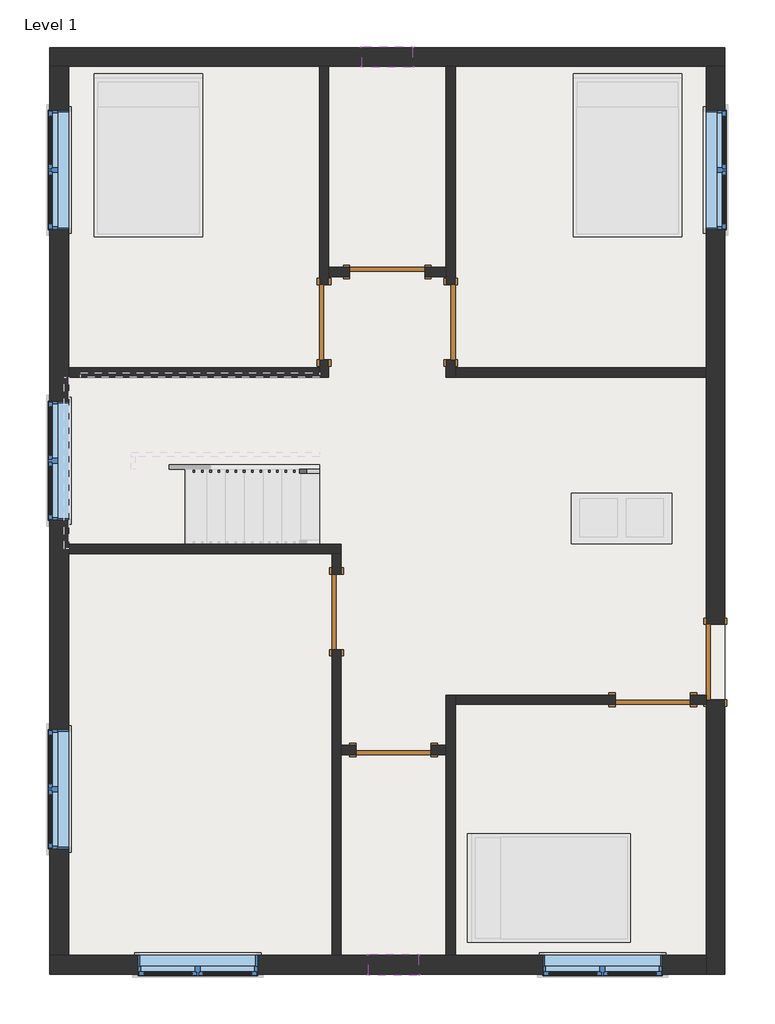
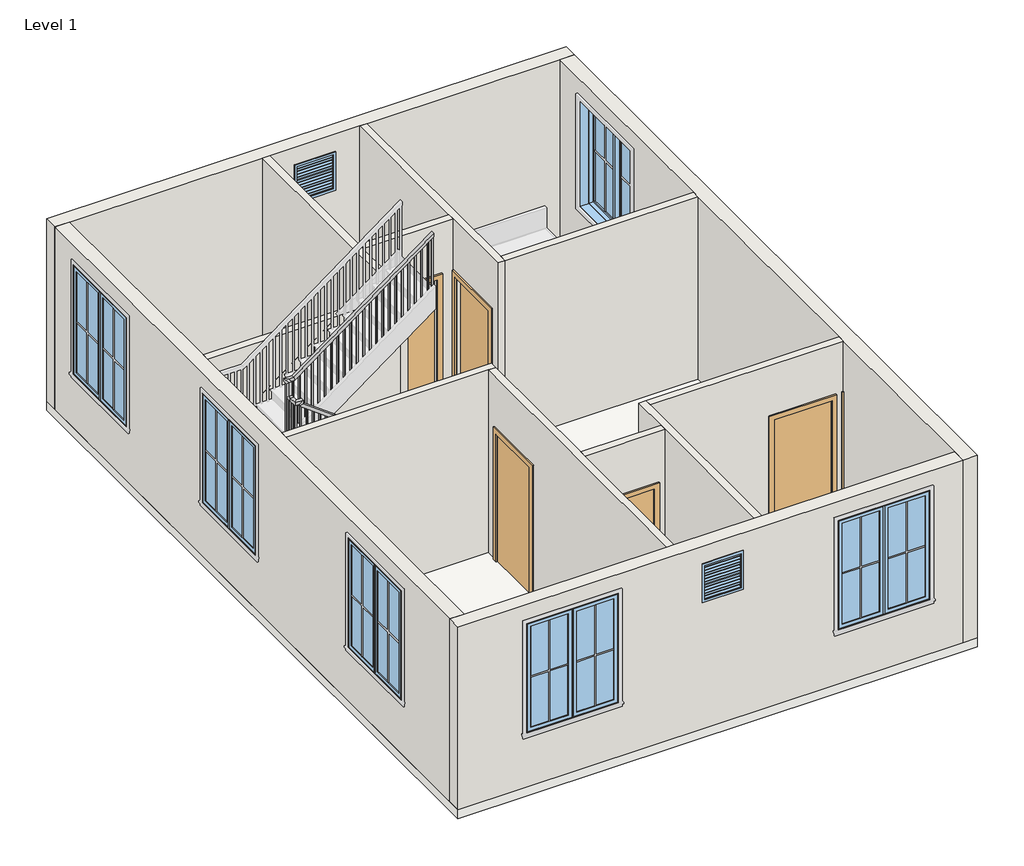
# One storey, part 1 of 2: 14 walls, 8 windows, 7 doors, 1 railing, 1 slab.
"""IFC4 building model written with IfcOpenShell, lengths in millimetres."""

from ifc_helpers import new_model, si_unit, frame, origin, origin_with_axes, place, context, project, spatial, polyline, outline, extrude, faceted_brep, transform, mapped, element, save
from components import door_305aa2a5, door_e5f9f3c4, door_0ca8825f, window_9ac97e1a, window_f2d8fef0

model = new_model("IFC4")

# Units and contexts
model_context = context("Model", 3, world=origin())
ifc_project = project(units=[si_unit("LENGTHUNIT", "METRE", prefix="MILLI")], contexts=[model_context])

# Site, building, storey
site = spatial("IfcSite", under=ifc_project)
building = spatial("IfcBuilding", under=site)
storey = spatial("IfcBuildingStorey", under=building, Name="Level 1", Elevation=0.0)

# Doors
placement = place(None, origin())
door_shape = door_305aa2a5(model_context)
element("IfcDoor", 1, ObjectType="Single-Flush : 36\" x 84\"", at=placement, inside=storey, context=model_context, shape_type="MappedRepresentation", body=[
    mapped(door_shape, transform((-2023.6910855, 2116.5303617, 0.0), x_axis=(0.0, -1.0, 0.0), y_axis=(1.0, 0.0, 0.0), z_axis=(0.0, 0.0, 1.0))),
])
element("IfcDoor", 2, ObjectType="Single-Flush : 36\" x 84\"", at=placement, inside=storey, context=model_context, shape_type="MappedRepresentation", body=[
    mapped(door_shape, transform((-1179.1410855, -3078.1725945, 0.0), x_axis=(1.0, 0.0, 0.0), y_axis=(0.0, 1.0, 0.0), z_axis=(0.0, 0.0, 1.0))),
])
element("IfcDoor", 3, ObjectType="Single-Flush : 36\" x 84\"", at=placement, inside=storey, context=model_context, shape_type="MappedRepresentation", body=[
    mapped(door_shape, transform((1970.4589145, -2468.1696383, 0.0), x_axis=(1.0, 0.0, 0.0), y_axis=(0.0, 1.0, 0.0), z_axis=(0.0, 0.0, 1.0))),
])
door_2_shape = door_e5f9f3c4(model_context)
element("IfcDoor", 4, ObjectType="Single-Flush : 36\" x 84\"", at=placement, inside=storey, context=model_context, shape_type="MappedRepresentation", body=[
    mapped(door_2_shape, transform((-486.9910855, 2116.5303617, 0.0), x_axis=(0.0, -1.0, 0.0), y_axis=(1.0, 0.0, 0.0), z_axis=(0.0, 0.0, 1.0))),
])
element("IfcDoor", 5, ObjectType="Single-Flush : 36\" x 84\"", at=placement, inside=storey, context=model_context, shape_type="MappedRepresentation", body=[
    mapped(door_2_shape, transform((-1871.2910855, -1401.3696383, 0.0), x_axis=(0.0, 1.0, 0.0), y_axis=(-1.0, 0.0, 0.0), z_axis=(0.0, 0.0, 1.0))),
])
element("IfcDoor", 6, ObjectType="Single-Flush : 36\" x 84\"", at=placement, inside=storey, context=model_context, shape_type="MappedRepresentation", body=[
    mapped(door_2_shape, transform((-1255.3410855, 2726.1303617, 0.0), x_axis=(1.0, 0.0, 0.0), y_axis=(0.0, 1.0, 0.0), z_axis=(0.0, 0.0, 1.0))),
])
door_3_shape = door_0ca8825f(model_context)
element("IfcDoor", 7, ObjectType="Single-Flush : 36\" x 84\"", at=placement, inside=storey, context=model_context, shape_type="MappedRepresentation", body=[
    mapped(door_3_shape, transform((2732.4589145, -2010.9696383, 0.0), x_axis=(0.0, 1.0, 0.0), y_axis=(-1.0, 0.0, 0.0), z_axis=(0.0, 0.0, 1.0))),
])

# Railing
element("IfcRailing", 8, ObjectType="Handrail - Rectangular", at=placement, inside=storey, context=model_context, shape_type="SolidModel", body=[
    faceted_brep([(-2080.8410855, 281.3803617, 1083.7333333), (-2080.8410855, 281.3803617, 1020.5144356), (-2080.8410855, 332.1803617, 1020.5144356), (-2080.8410855, 332.1803617, 1083.7333333), (-4290.6410855, 281.3803617, 2720.6222222), (-4341.4410855, 281.3803617, 2695.0329542), (-4341.4410855, 332.1803617, 2695.0329542), (-4290.6410855, 332.1803617, 2720.6222222), (-4290.6410855, 281.3803617, 2777.0666667), (-4341.4410855, 281.3803617, 2726.2666667), (-4341.4410855, 332.1803617, 2726.2666667), (-4290.6410855, 332.1803617, 2777.0666667), (-4417.6410855, 281.3803617, 2777.0666667), (-4417.6410855, 281.3803617, 2726.2666667), (-4366.8410855, 332.1803617, 2726.2666667), (-4366.8410855, 332.1803617, 2777.0666667), (-4417.6410855, 408.3803617, 2777.0666667), (-4417.6410855, 408.3803617, 2726.2666667), (-4366.8410855, 408.3803617, 2726.2666667), (-4366.8410855, 408.3803617, 2777.0666667), (-4417.6410855, 459.1803617, 2777.0666667), (-4417.6410855, 509.9803617, 2726.2666667), (-4366.8410855, 509.9803617, 2726.2666667), (-4366.8410855, 459.1803617, 2777.0666667), (-4417.6410855, 459.1803617, 3002.8444444), (-4417.6410855, 509.9803617, 2952.0444444), (-4366.8410855, 509.9803617, 2952.0444444), (-4366.8410855, 459.1803617, 3002.8444444), (-4417.6410855, 586.1803617, 3002.8444444), (-4417.6410855, 586.1803617, 2952.0444444), (-4366.8410855, 535.3803617, 2952.0444444), (-4366.8410855, 535.3803617, 3002.8444444), (-4290.6410855, 586.1803617, 3002.8444444), (-4273.8755736, 586.1803617, 2952.0444444), (-4273.8755736, 535.3803617, 2952.0444444), (-4290.6410855, 535.3803617, 3002.8444444), (-2080.8410855, 586.1803617, 4639.7333333), (-2080.8410855, 535.3803617, 4639.7333333), (-2080.8410855, 535.3803617, 4576.5144356), (-2080.8410855, 586.1803617, 4576.5144356)], [[[0, 1, 2, 3]], [[1, 0, 4, 5]], [[2, 1, 5, 6]], [[3, 2, 6, 7]], [[0, 3, 7, 4]], [[5, 4, 8, 9]], [[6, 5, 9, 10]], [[7, 6, 10, 11]], [[4, 7, 11, 8]], [[9, 8, 12, 13]], [[10, 9, 13, 14]], [[11, 10, 14, 15]], [[8, 11, 15, 12]], [[13, 12, 16, 17]], [[14, 13, 17, 18]], [[15, 14, 18, 19]], [[12, 15, 19, 16]], [[17, 16, 20, 21]], [[18, 17, 21, 22]], [[19, 18, 22, 23]], [[16, 19, 23, 20]], [[21, 20, 24, 25]], [[22, 21, 25, 26]], [[23, 22, 26, 27]], [[20, 23, 27, 24]], [[25, 24, 28, 29]], [[26, 25, 29, 30]], [[27, 26, 30, 31]], [[24, 27, 31, 28]], [[29, 28, 32, 33]], [[30, 29, 33, 34]], [[31, 30, 34, 35]], [[28, 31, 35, 32]], [[36, 37, 38, 39]], [[33, 32, 36, 39]], [[34, 33, 39, 38]], [[35, 34, 38, 37]], [[32, 35, 37, 36]]]),
    extrude(outline(polyline([(4527.1255467, -2147.5160855), (4513.0144356, -2166.5660855), (3556.0, -2166.5660855), (3556.0, -2147.5160855), (4527.1255467, -2147.5160855)])), frame((0.0, 551.2553617, 0.0), z_axis=(0.0, 1.0, 0.0), x_axis=(0.0, 0.0, 1.0)), (0.0, 0.0, 1.0), 19.05),
    extrude(outline(polyline([(4451.8662875, -2249.1160855), (4437.7551764, -2268.1660855), (3556.0, -2268.1660855), (3556.0, -2249.1160855), (4451.8662875, -2249.1160855)])), frame((0.0, 551.2553617, 0.0), z_axis=(0.0, 1.0, 0.0), x_axis=(0.0, 0.0, 1.0)), (0.0, 0.0, 1.0), 19.05),
    extrude(outline(polyline([(4376.6070282, -2350.7160855), (4362.4959171, -2369.7660855), (3386.6666667, -2369.7660855), (3386.6666667, -2350.7160855), (4376.6070282, -2350.7160855)])), frame((0.0, 551.2553617, 0.0), z_axis=(0.0, 1.0, 0.0), x_axis=(0.0, 0.0, 1.0)), (0.0, 0.0, 1.0), 19.05),
    extrude(outline(polyline([(4301.347769, -2452.3160855), (4287.2366579, -2471.3660855), (3386.6666667, -2471.3660855), (3386.6666667, -2452.3160855), (4301.347769, -2452.3160855)])), frame((0.0, 551.2553617, 0.0), z_axis=(0.0, 1.0, 0.0), x_axis=(0.0, 0.0, 1.0)), (0.0, 0.0, 1.0), 19.05),
    extrude(outline(polyline([(4226.0885097, -2553.9160855), (4211.9773986, -2572.9660855), (3217.3333333, -2572.9660855), (3217.3333333, -2553.9160855), (4226.0885097, -2553.9160855)])), frame((0.0, 551.2553617, 0.0), z_axis=(0.0, 1.0, 0.0), x_axis=(0.0, 0.0, 1.0)), (0.0, 0.0, 1.0), 19.05),
    extrude(outline(polyline([(4150.8292505, -2655.5160855), (4136.7181393, -2674.5660855), (3217.3333333, -2674.5660855), (3217.3333333, -2655.5160855), (4150.8292505, -2655.5160855)])), frame((0.0, 551.2553617, 0.0), z_axis=(0.0, 1.0, 0.0), x_axis=(0.0, 0.0, 1.0)), (0.0, 0.0, 1.0), 19.05),
    extrude(outline(polyline([(4075.5699912, -2757.1160855), (4061.4588801, -2776.1660855), (3217.3333333, -2776.1660855), (3217.3333333, -2757.1160855), (4075.5699912, -2757.1160855)])), frame((0.0, 551.2553617, 0.0), z_axis=(0.0, 1.0, 0.0), x_axis=(0.0, 0.0, 1.0)), (0.0, 0.0, 1.0), 19.05),
    extrude(outline(polyline([(4000.3107319, -2858.7160855), (3986.1996208, -2877.7660855), (3048.0, -2877.7660855), (3048.0, -2858.7160855), (4000.3107319, -2858.7160855)])), frame((0.0, 551.2553617, 0.0), z_axis=(0.0, 1.0, 0.0), x_axis=(0.0, 0.0, 1.0)), (0.0, 0.0, 1.0), 19.05),
    extrude(outline(polyline([(3925.0514727, -2960.3160855), (3910.9403616, -2979.3660855), (3048.0, -2979.3660855), (3048.0, -2960.3160855), (3925.0514727, -2960.3160855)])), frame((0.0, 551.2553617, 0.0), z_axis=(0.0, 1.0, 0.0), x_axis=(0.0, 0.0, 1.0)), (0.0, 0.0, 1.0), 19.05),
    extrude(outline(polyline([(3849.7922134, -3061.9160855), (3835.6811023, -3080.9660855), (2878.6666667, -3080.9660855), (2878.6666667, -3061.9160855), (3849.7922134, -3061.9160855)])), frame((0.0, 551.2553617, 0.0), z_axis=(0.0, 1.0, 0.0), x_axis=(0.0, 0.0, 1.0)), (0.0, 0.0, 1.0), 19.05),
    extrude(outline(polyline([(3774.5329542, -3163.5160855), (3760.421843, -3182.5660855), (2878.6666667, -3182.5660855), (2878.6666667, -3163.5160855), (3774.5329542, -3163.5160855)])), frame((0.0, 551.2553617, 0.0), z_axis=(0.0, 1.0, 0.0), x_axis=(0.0, 0.0, 1.0)), (0.0, 0.0, 1.0), 19.05),
    extrude(outline(polyline([(3699.2736949, -3265.1160855), (3685.1625838, -3284.1660855), (2709.3333333, -3284.1660855), (2709.3333333, -3265.1160855), (3699.2736949, -3265.1160855)])), frame((0.0, 551.2553617, 0.0), z_axis=(0.0, 1.0, 0.0), x_axis=(0.0, 0.0, 1.0)), (0.0, 0.0, 1.0), 19.05),
    extrude(outline(polyline([(3624.0144356, -3366.7160855), (3609.9033245, -3385.7660855), (2709.3333333, -3385.7660855), (2709.3333333, -3366.7160855), (3624.0144356, -3366.7160855)])), frame((0.0, 551.2553617, 0.0), z_axis=(0.0, 1.0, 0.0), x_axis=(0.0, 0.0, 1.0)), (0.0, 0.0, 1.0), 19.05),
    extrude(outline(polyline([(3548.7551764, -3468.3160855), (3534.6440653, -3487.3660855), (2540.0, -3487.3660855), (2540.0, -3468.3160855), (3548.7551764, -3468.3160855)])), frame((0.0, 551.2553617, 0.0), z_axis=(0.0, 1.0, 0.0), x_axis=(0.0, 0.0, 1.0)), (0.0, 0.0, 1.0), 19.05),
    extrude(outline(polyline([(3473.4959171, -3569.9160855), (3459.384806, -3588.9660855), (2540.0, -3588.9660855), (2540.0, -3569.9160855), (3473.4959171, -3569.9160855)])), frame((0.0, 551.2553617, 0.0), z_axis=(0.0, 1.0, 0.0), x_axis=(0.0, 0.0, 1.0)), (0.0, 0.0, 1.0), 19.05),
    extrude(outline(polyline([(3398.2366579, -3671.5160855), (3384.1255467, -3690.5660855), (2540.0, -3690.5660855), (2540.0, -3671.5160855), (3398.2366579, -3671.5160855)])), frame((0.0, 551.2553617, 0.0), z_axis=(0.0, 1.0, 0.0), x_axis=(0.0, 0.0, 1.0)), (0.0, 0.0, 1.0), 19.05),
    extrude(outline(polyline([(3322.9773986, -3773.1160855), (3308.8662875, -3792.1660855), (2370.6666667, -3792.1660855), (2370.6666667, -3773.1160855), (3322.9773986, -3773.1160855)])), frame((0.0, 551.2553617, 0.0), z_axis=(0.0, 1.0, 0.0), x_axis=(0.0, 0.0, 1.0)), (0.0, 0.0, 1.0), 19.05),
    extrude(outline(polyline([(3247.7181393, -3874.7160855), (3233.6070282, -3893.7660855), (2370.6666667, -3893.7660855), (2370.6666667, -3874.7160855), (3247.7181393, -3874.7160855)])), frame((0.0, 551.2553617, 0.0), z_axis=(0.0, 1.0, 0.0), x_axis=(0.0, 0.0, 1.0)), (0.0, 0.0, 1.0), 19.05),
    extrude(outline(polyline([(3172.4588801, -3976.3160855), (3158.347769, -3995.3660855), (2201.3333333, -3995.3660855), (2201.3333333, -3976.3160855), (3172.4588801, -3976.3160855)])), frame((0.0, 551.2553617, 0.0), z_axis=(0.0, 1.0, 0.0), x_axis=(0.0, 0.0, 1.0)), (0.0, 0.0, 1.0), 19.05),
    extrude(outline(polyline([(3097.1996208, -4077.9160855), (3083.0885097, -4096.9660855), (2201.3333333, -4096.9660855), (2201.3333333, -4077.9160855), (3097.1996208, -4077.9160855)])), frame((0.0, 551.2553617, 0.0), z_axis=(0.0, 1.0, 0.0), x_axis=(0.0, 0.0, 1.0)), (0.0, 0.0, 1.0), 19.05),
    extrude(outline(polyline([(3021.9403616, -4179.5160855), (3007.8292505, -4198.5660855), (2032.0, -4198.5660855), (2032.0, -4179.5160855), (3021.9403616, -4179.5160855)])), frame((0.0, 551.2553617, 0.0), z_axis=(0.0, 1.0, 0.0), x_axis=(0.0, 0.0, 1.0)), (0.0, 0.0, 1.0), 19.05),
    extrude(outline(polyline([(2946.6811023, -4281.1160855), (2932.5699912, -4300.1660855), (2032.0, -4300.1660855), (2032.0, -4281.1160855), (2946.6811023, -4281.1160855)])), frame((0.0, 551.2553617, 0.0), z_axis=(0.0, 1.0, 0.0), x_axis=(0.0, 0.0, 1.0)), (0.0, 0.0, 1.0), 19.05),
    extrude(outline(polyline([(-4382.7160855, 500.4553617), (-4401.7660855, 500.4553617), (-4401.7660855, 519.5053617), (-4382.7160855, 519.5053617), (-4382.7160855, 500.4553617)])), frame((0.0, 0.0, 1862.6666667), z_axis=(0.0, 0.0, 1.0), x_axis=(1.0, 0.0, 0.0)), (0.0, 0.0, 1.0), 1089.3777778),
    extrude(outline(polyline([(-4382.7160855, 398.8553617), (-4401.7660855, 398.8553617), (-4401.7660855, 417.9053617), (-4382.7160855, 417.9053617), (-4382.7160855, 398.8553617)])), frame((0.0, 0.0, 1862.6666667), z_axis=(0.0, 0.0, 1.0), x_axis=(1.0, 0.0, 0.0)), (0.0, 0.0, 1.0), 863.6),
    extrude(outline(polyline([(-4306.5160855, 316.3053617), (-4306.5160855, 297.2553617), (-4325.5660855, 297.2553617), (-4325.5660855, 316.3053617), (-4306.5160855, 316.3053617)])), frame((0.0, 0.0, 1693.3333333), z_axis=(0.0, 0.0, 1.0), x_axis=(1.0, 0.0, 0.0)), (0.0, 0.0, 1.0), 1032.9333333),
    extrude(outline(polyline([(2593.9033245, -4204.9160855), (2608.0144356, -4223.9660855), (1693.3333333, -4223.9660855), (1693.3333333, -4204.9160855), (2593.9033245, -4204.9160855)])), frame((0.0, 297.2553617, 0.0), z_axis=(0.0, 1.0, 0.0), x_axis=(0.0, 0.0, 1.0)), (0.0, 0.0, 1.0), 19.05),
    extrude(outline(polyline([(2518.6440653, -4103.3160855), (2532.7551764, -4122.3660855), (1524.0, -4122.3660855), (1524.0, -4103.3160855), (2518.6440653, -4103.3160855)])), frame((0.0, 297.2553617, 0.0), z_axis=(0.0, 1.0, 0.0), x_axis=(0.0, 0.0, 1.0)), (0.0, 0.0, 1.0), 19.05),
    extrude(outline(polyline([(2443.384806, -4001.7160855), (2457.4959171, -4020.7660855), (1524.0, -4020.7660855), (1524.0, -4001.7160855), (2443.384806, -4001.7160855)])), frame((0.0, 297.2553617, 0.0), z_axis=(0.0, 1.0, 0.0), x_axis=(0.0, 0.0, 1.0)), (0.0, 0.0, 1.0), 19.05),
    extrude(outline(polyline([(2368.1255467, -3900.1160855), (2382.2366579, -3919.1660855), (1524.0, -3919.1660855), (1524.0, -3900.1160855), (2368.1255467, -3900.1160855)])), frame((0.0, 297.2553617, 0.0), z_axis=(0.0, 1.0, 0.0), x_axis=(0.0, 0.0, 1.0)), (0.0, 0.0, 1.0), 19.05),
    extrude(outline(polyline([(2292.8662875, -3798.5160855), (2306.9773986, -3817.5660855), (1354.6666667, -3817.5660855), (1354.6666667, -3798.5160855), (2292.8662875, -3798.5160855)])), frame((0.0, 297.2553617, 0.0), z_axis=(0.0, 1.0, 0.0), x_axis=(0.0, 0.0, 1.0)), (0.0, 0.0, 1.0), 19.05),
    extrude(outline(polyline([(2217.6070282, -3696.9160855), (2231.7181393, -3715.9660855), (1354.6666667, -3715.9660855), (1354.6666667, -3696.9160855), (2217.6070282, -3696.9160855)])), frame((0.0, 297.2553617, 0.0), z_axis=(0.0, 1.0, 0.0), x_axis=(0.0, 0.0, 1.0)), (0.0, 0.0, 1.0), 19.05),
    extrude(outline(polyline([(2142.347769, -3595.3160855), (2156.4588801, -3614.3660855), (1185.3333333, -3614.3660855), (1185.3333333, -3595.3160855), (2142.347769, -3595.3160855)])), frame((0.0, 297.2553617, 0.0), z_axis=(0.0, 1.0, 0.0), x_axis=(0.0, 0.0, 1.0)), (0.0, 0.0, 1.0), 19.05),
    extrude(outline(polyline([(2067.0885097, -3493.7160855), (2081.1996208, -3512.7660855), (1185.3333333, -3512.7660855), (1185.3333333, -3493.7160855), (2067.0885097, -3493.7160855)])), frame((0.0, 297.2553617, 0.0), z_axis=(0.0, 1.0, 0.0), x_axis=(0.0, 0.0, 1.0)), (0.0, 0.0, 1.0), 19.05),
    extrude(outline(polyline([(1991.8292505, -3392.1160855), (2005.9403616, -3411.1660855), (1016.0, -3411.1660855), (1016.0, -3392.1160855), (1991.8292505, -3392.1160855)])), frame((0.0, 297.2553617, 0.0), z_axis=(0.0, 1.0, 0.0), x_axis=(0.0, 0.0, 1.0)), (0.0, 0.0, 1.0), 19.05),
    extrude(outline(polyline([(1916.5699912, -3290.5160855), (1930.6811023, -3309.5660855), (1016.0, -3309.5660855), (1016.0, -3290.5160855), (1916.5699912, -3290.5160855)])), frame((0.0, 297.2553617, 0.0), z_axis=(0.0, 1.0, 0.0), x_axis=(0.0, 0.0, 1.0)), (0.0, 0.0, 1.0), 19.05),
    extrude(outline(polyline([(1841.3107319, -3188.9160855), (1855.421843, -3207.9660855), (846.6666667, -3207.9660855), (846.6666667, -3188.9160855), (1841.3107319, -3188.9160855)])), frame((0.0, 297.2553617, 0.0), z_axis=(0.0, 1.0, 0.0), x_axis=(0.0, 0.0, 1.0)), (0.0, 0.0, 1.0), 19.05),
    extrude(outline(polyline([(1766.0514727, -3087.3160855), (1780.1625838, -3106.3660855), (846.6666667, -3106.3660855), (846.6666667, -3087.3160855), (1766.0514727, -3087.3160855)])), frame((0.0, 297.2553617, 0.0), z_axis=(0.0, 1.0, 0.0), x_axis=(0.0, 0.0, 1.0)), (0.0, 0.0, 1.0), 19.05),
    extrude(outline(polyline([(1690.7922134, -2985.7160855), (1704.9033245, -3004.7660855), (846.6666667, -3004.7660855), (846.6666667, -2985.7160855), (1690.7922134, -2985.7160855)])), frame((0.0, 297.2553617, 0.0), z_axis=(0.0, 1.0, 0.0), x_axis=(0.0, 0.0, 1.0)), (0.0, 0.0, 1.0), 19.05),
    extrude(outline(polyline([(1615.5329542, -2884.1160855), (1629.6440653, -2903.1660855), (677.3333333, -2903.1660855), (677.3333333, -2884.1160855), (1615.5329542, -2884.1160855)])), frame((0.0, 297.2553617, 0.0), z_axis=(0.0, 1.0, 0.0), x_axis=(0.0, 0.0, 1.0)), (0.0, 0.0, 1.0), 19.05),
    extrude(outline(polyline([(1540.2736949, -2782.5160855), (1554.384806, -2801.5660855), (677.3333333, -2801.5660855), (677.3333333, -2782.5160855), (1540.2736949, -2782.5160855)])), frame((0.0, 297.2553617, 0.0), z_axis=(0.0, 1.0, 0.0), x_axis=(0.0, 0.0, 1.0)), (0.0, 0.0, 1.0), 19.05),
    extrude(outline(polyline([(1465.0144356, -2680.9160855), (1479.1255467, -2699.9660855), (508.0, -2699.9660855), (508.0, -2680.9160855), (1465.0144356, -2680.9160855)])), frame((0.0, 297.2553617, 0.0), z_axis=(0.0, 1.0, 0.0), x_axis=(0.0, 0.0, 1.0)), (0.0, 0.0, 1.0), 19.05),
    extrude(outline(polyline([(1389.7551764, -2579.3160855), (1403.8662875, -2598.3660855), (508.0, -2598.3660855), (508.0, -2579.3160855), (1389.7551764, -2579.3160855)])), frame((0.0, 297.2553617, 0.0), z_axis=(0.0, 1.0, 0.0), x_axis=(0.0, 0.0, 1.0)), (0.0, 0.0, 1.0), 19.05),
    extrude(outline(polyline([(1314.4959171, -2477.7160855), (1328.6070282, -2496.7660855), (338.6666667, -2496.7660855), (338.6666667, -2477.7160855), (1314.4959171, -2477.7160855)])), frame((0.0, 297.2553617, 0.0), z_axis=(0.0, 1.0, 0.0), x_axis=(0.0, 0.0, 1.0)), (0.0, 0.0, 1.0), 19.05),
    extrude(outline(polyline([(1239.2366579, -2376.1160855), (1253.347769, -2395.1660855), (338.6666667, -2395.1660855), (338.6666667, -2376.1160855), (1239.2366579, -2376.1160855)])), frame((0.0, 297.2553617, 0.0), z_axis=(0.0, 1.0, 0.0), x_axis=(0.0, 0.0, 1.0)), (0.0, 0.0, 1.0), 19.05),
    extrude(outline(polyline([(1163.9773986, -2274.5160855), (1178.0885097, -2293.5660855), (169.3333333, -2293.5660855), (169.3333333, -2274.5160855), (1163.9773986, -2274.5160855)])), frame((0.0, 297.2553617, 0.0), z_axis=(0.0, 1.0, 0.0), x_axis=(0.0, 0.0, 1.0)), (0.0, 0.0, 1.0), 19.05),
    extrude(outline(polyline([(1088.7181393, -2172.9160855), (1102.8292505, -2191.9660855), (169.3333333, -2191.9660855), (169.3333333, -2172.9160855), (1088.7181393, -2172.9160855)])), frame((0.0, 297.2553617, 0.0), z_axis=(0.0, 1.0, 0.0), x_axis=(0.0, 0.0, 1.0)), (0.0, 0.0, 1.0), 19.05),
    extrude(outline(polyline([(-4382.7160855, 551.2553617), (-4401.7660855, 551.2553617), (-4401.7660855, 570.3053617), (-4382.7160855, 570.3053617), (-4382.7160855, 551.2553617)])), frame((0.0, 0.0, 1862.6666667), z_axis=(0.0, 0.0, 1.0), x_axis=(1.0, 0.0, 0.0)), (0.0, 0.0, 1.0), 1089.3777778),
    extrude(outline(polyline([(-4382.7160855, 316.3053617), (-4382.7160855, 297.2553617), (-4401.7660855, 297.2553617), (-4401.7660855, 316.3053617), (-4382.7160855, 316.3053617)])), frame((0.0, 0.0, 1862.6666667), z_axis=(0.0, 0.0, 1.0), x_axis=(1.0, 0.0, 0.0)), (0.0, 0.0, 1.0), 863.6),
    extrude(outline(polyline([(4576.5144356, -2080.8410855), (4562.4033245, -2099.8910855), (3556.0, -2099.8910855), (3556.0, -2080.8410855), (4576.5144356, -2080.8410855)])), frame((0.0, 551.2553617, 0.0), z_axis=(0.0, 1.0, 0.0), x_axis=(0.0, 0.0, 1.0)), (0.0, 0.0, 1.0), 19.05),
    extrude(outline(polyline([(1020.5144356, -2080.8410855), (1034.6255467, -2099.8910855), (169.3333333, -2099.8910855), (169.3333333, -2080.8410855), (1020.5144356, -2080.8410855)])), frame((0.0, 297.2553617, 0.0), z_axis=(0.0, 1.0, 0.0), x_axis=(0.0, 0.0, 1.0)), (0.0, 0.0, 1.0), 19.05),
])

# Slab
element("IfcSlab", 9, ObjectType="FLOOR 6\"", at=placement, inside=storey, context=model_context, shape_type="SweptSolid", body=[
    extrude(outline(polyline([(2846.7589145, 5450.2803617), (2846.7589145, -5801.9196383), (-5357.4410855, -5801.9196383), (-5357.4410855, 5450.2803617), (2846.7589145, 5450.2803617)])), frame((0.0, 0.0, -152.4), z_axis=(0.0, 0.0, 1.0), x_axis=(1.0, 0.0, 0.0)), (0.0, 0.0, 1.0), 152.4),
])

# Walls
element("IfcWall", 10, ObjectType="WALL 4.5\"", at=placement, inside=storey, context=model_context, shape_type="Brep", body=[
    faceted_brep([(-2080.8410855, 1659.3303617, 2133.6), (-2080.8410855, 1659.3303617, 0.0), (-2080.8410855, 1564.0803617, 0.0), (-2080.8410855, 1449.7803617, 0.0), (-2080.8410855, 1449.7803617, 3048.0), (-2080.8410855, 1564.0803617, 3048.0), (-2080.8410855, 5221.6803617, 3048.0), (-2080.8410855, 5221.6803617, 0.0), (-2080.8410855, 2573.7303617, 0.0), (-2080.8410855, 2573.7303617, 2133.6), (-1966.5410855, 1449.7803617, 0.0), (-1966.5410855, 1659.3303617, 0.0), (-1966.5410855, 1659.3303617, 2133.6), (-1966.5410855, 2573.7303617, 2133.6), (-1966.5410855, 2573.7303617, 0.0), (-1966.5410855, 2668.9803617, 0.0), (-1966.5410855, 2783.2803617, 0.0), (-1966.5410855, 5221.6803617, 0.0), (-1966.5410855, 5221.6803617, 3048.0), (-1966.5410855, 2783.2803617, 3048.0), (-1966.5410855, 2668.9803617, 3048.0), (-1966.5410855, 1449.7803617, 3048.0)], [[[0, 1, 2, 3, 4, 5, 6, 7, 8, 9]], [[10, 11, 12, 13, 14, 15, 16, 17, 18, 19, 20, 21]], [[8, 7, 17, 16, 15, 14]], [[3, 2, 1, 11, 10]], [[7, 6, 18, 17]], [[4, 3, 10, 21]], [[12, 11, 1, 0]], [[13, 12, 0, 9]], [[14, 13, 9, 8]], [[6, 5, 4, 21, 20, 19, 18]]]),
])
element("IfcWall", 11, ObjectType="WALL 4.5\"", at=placement, inside=storey, context=model_context, shape_type="SweptSolid", body=[
    extrude(outline(polyline([(-5128.8410855, 1564.0803617), (-2080.8410855, 1564.0803617), (-2080.8410855, 1449.7803617), (-5128.8410855, 1449.7803617), (-5128.8410855, 1564.0803617)])), origin_with_axes(), (0.0, 0.0, 1.0), 3048.0),
])
element("IfcWall", 12, ObjectType="WALL 4.5\"", at=placement, inside=storey, context=model_context, shape_type="Brep", body=[
    faceted_brep([(-544.1410855, 1659.3303617, 2133.6), (-544.1410855, 1659.3303617, 0.0), (-544.1410855, 1449.7803617, 0.0), (-544.1410855, 1449.7803617, 3048.0), (-544.1410855, 2668.9803617, 3048.0), (-544.1410855, 2783.2803617, 3048.0), (-544.1410855, 5221.6803617, 3048.0), (-544.1410855, 5221.6803617, 0.0), (-544.1410855, 2783.2803617, 0.0), (-544.1410855, 2668.9803617, 0.0), (-544.1410855, 2573.7303617, 0.0), (-544.1410855, 2573.7303617, 2133.6), (-429.8410855, 1449.7803617, 0.0), (-429.8410855, 1564.0803617, 0.0), (-429.8410855, 1659.3303617, 0.0), (-429.8410855, 1659.3303617, 2133.6), (-429.8410855, 2573.7303617, 2133.6), (-429.8410855, 2573.7303617, 0.0), (-429.8410855, 5221.6803617, 0.0), (-429.8410855, 5221.6803617, 3048.0), (-429.8410855, 1564.0803617, 3048.0), (-429.8410855, 1449.7803617, 3048.0)], [[[0, 1, 2, 3, 4, 5, 6, 7, 8, 9, 10, 11]], [[12, 13, 14, 15, 16, 17, 18, 19, 20, 21]], [[2, 1, 14, 13, 12]], [[10, 9, 8, 7, 18, 17]], [[7, 6, 19, 18]], [[3, 2, 12, 21]], [[15, 14, 1, 0]], [[16, 15, 0, 11]], [[17, 16, 11, 10]], [[6, 5, 4, 3, 21, 20, 19]]]),
])
element("IfcWall", 13, ObjectType="WALL 4.5\"", at=placement, inside=storey, context=model_context, shape_type="SweptSolid", body=[
    extrude(outline(polyline([(2618.1589145, 1449.7803617), (-429.8410855, 1449.7803617), (-429.8410855, 1564.0803617), (2618.1589145, 1564.0803617), (2618.1589145, 1449.7803617)])), origin_with_axes(), (0.0, 0.0, 1.0), 3048.0),
])
element("IfcWall", 14, ObjectType="WALL 4.5\"", at=placement, inside=storey, context=model_context, shape_type="Brep", body=[
    faceted_brep([(-5128.8410855, -696.5196383, 0.0), (-1928.4410855, -696.5196383, 0.0), (-1814.1410855, -696.5196383, 0.0), (-1814.1410855, -696.5196383, 3048.0), (-1928.4410855, -696.5196383, 3048.0), (-5128.8410855, -696.5196383, 3048.0), (-5128.8410855, -582.2196383, 0.0), (-5128.8410855, -582.2196383, 3048.0), (-1814.1410855, -582.2196383, 3048.0), (-1814.1410855, -582.2196383, 0.0)], [[[0, 1, 2, 3, 4, 5]], [[6, 7, 8, 9]], [[2, 1, 0, 6, 9]], [[0, 5, 7, 6]], [[3, 2, 9, 8]], [[5, 4, 3, 8, 7]]]),
])
element("IfcWall", 15, ObjectType="WALL 4.5\"", at=placement, inside=storey, context=model_context, shape_type="Brep", body=[
    faceted_brep([(-1814.1410855, -944.1696383, 2133.6), (-1814.1410855, -944.1696383, 0.0), (-1814.1410855, -696.5196383, 0.0), (-1814.1410855, -696.5196383, 3048.0), (-1814.1410855, -3021.0225945, 3048.0), (-1814.1410855, -3135.3225945, 3048.0), (-1814.1410855, -5573.3196383, 3048.0), (-1814.1410855, -5573.3196383, 0.0), (-1814.1410855, -3135.3225945, 0.0), (-1814.1410855, -3021.0225945, 0.0), (-1814.1410855, -1858.5696383, 0.0), (-1814.1410855, -1858.5696383, 2133.6), (-1928.4410855, -696.5196383, 0.0), (-1928.4410855, -944.1696383, 0.0), (-1928.4410855, -944.1696383, 2133.6), (-1928.4410855, -1858.5696383, 2133.6), (-1928.4410855, -1858.5696383, 0.0), (-1928.4410855, -5573.3196383, 0.0), (-1928.4410855, -5573.3196383, 3048.0), (-1928.4410855, -696.5196383, 3048.0)], [[[0, 1, 2, 3, 4, 5, 6, 7, 8, 9, 10, 11]], [[12, 13, 14, 15, 16, 17, 18, 19]], [[2, 1, 13, 12]], [[10, 9, 8, 7, 17, 16]], [[3, 2, 12, 19]], [[7, 6, 18, 17]], [[14, 13, 1, 0]], [[15, 14, 0, 11]], [[16, 15, 11, 10]], [[6, 5, 4, 3, 19, 18]]]),
])
element("IfcWall", 16, ObjectType="WALL 4.5\"", at=placement, inside=storey, context=model_context, shape_type="SweptSolid", body=[
    extrude(outline(polyline([(2133.6, -721.9410855), (0.0, -721.9410855), (0.0, -544.1410855), (3048.0, -544.1410855), (3048.0, -1814.1410855), (0.0, -1814.1410855), (0.0, -1636.3410855), (2133.6, -1636.3410855), (2133.6, -721.9410855)])), frame((0.0, -3135.3225945, 0.0), z_axis=(0.0, 1.0, 0.0), x_axis=(0.0, 0.0, 1.0)), (0.0, 0.0, 1.0), 114.3),
])
element("IfcWall", 17, ObjectType="WALL 4.5\"", at=placement, inside=storey, context=model_context, shape_type="Brep", body=[
    faceted_brep([(-544.1410855, -2411.0196383, 0.0), (-544.1410855, -3021.0225945, 0.0), (-544.1410855, -3135.3225945, 0.0), (-544.1410855, -5573.3196383, 0.0), (-544.1410855, -5573.3196383, 3048.0), (-544.1410855, -3135.3225945, 3048.0), (-544.1410855, -3021.0225945, 3048.0), (-544.1410855, -2411.0196383, 3048.0), (-429.8410855, -2411.0196383, 0.0), (-429.8410855, -2411.0196383, 3048.0), (-429.8410855, -2525.3196383, 3048.0), (-429.8410855, -5573.3196383, 3048.0), (-429.8410855, -5573.3196383, 0.0), (-429.8410855, -2525.3196383, 0.0)], [[[0, 1, 2, 3, 4, 5, 6, 7]], [[8, 9, 10, 11, 12, 13]], [[3, 2, 1, 0, 8, 13, 12]], [[4, 3, 12, 11]], [[0, 7, 9, 8]], [[7, 6, 5, 4, 11, 10, 9]]]),
])
element("IfcWall", 18, ObjectType="WALL 4.5\"", at=placement, inside=storey, context=model_context, shape_type="Brep", body=[
    faceted_brep([(2427.6589145, -2525.3196383, 2133.6), (2427.6589145, -2525.3196383, 0.0), (2618.1589145, -2525.3196383, 0.0), (2618.1589145, -2525.3196383, 3048.0), (-429.8410855, -2525.3196383, 3048.0), (-429.8410855, -2525.3196383, 0.0), (1513.2589145, -2525.3196383, 0.0), (1513.2589145, -2525.3196383, 2133.6), (2618.1589145, -2411.0196383, 0.0), (2427.6589145, -2411.0196383, 0.0), (2427.6589145, -2411.0196383, 2133.6), (1513.2589145, -2411.0196383, 2133.6), (1513.2589145, -2411.0196383, 0.0), (-429.8410855, -2411.0196383, 0.0), (-429.8410855, -2411.0196383, 3048.0), (2618.1589145, -2411.0196383, 3048.0), (2618.1589145, -2468.1696383, 0.0)], [[[0, 1, 2, 3, 4, 5, 6, 7]], [[8, 9, 10, 11, 12, 13, 14, 15]], [[6, 5, 13, 12]], [[2, 1, 9, 8, 16]], [[5, 4, 14, 13]], [[3, 2, 16, 8, 15]], [[10, 9, 1, 0]], [[11, 10, 0, 7]], [[12, 11, 7, 6]], [[4, 3, 15, 14]]]),
])
element("IfcWall", 19, ObjectType="WALL 4.5\"", at=placement, inside=storey, context=model_context, shape_type="SweptSolid", body=[
    extrude(outline(polyline([(2133.6, -798.1410855), (0.0, -798.1410855), (0.0, -544.1410855), (3048.0, -544.1410855), (3048.0, -1966.5410855), (0.0, -1966.5410855), (0.0, -1712.5410855), (2133.6, -1712.5410855), (2133.6, -798.1410855)])), frame((0.0, 2668.9803617, 0.0), z_axis=(0.0, 1.0, 0.0), x_axis=(0.0, 0.0, 1.0)), (0.0, 0.0, 1.0), 114.3),
])
element("IfcWall", 20, ObjectType="WALL 9\"", at=placement, inside=storey, context=model_context, shape_type="Brep", body=[
    faceted_brep([(-5357.4410855, 5221.6803617, 0.0), (-5128.8410855, 5221.6803617, 0.0), (-2080.8410855, 5221.6803617, 0.0), (-1966.5410855, 5221.6803617, 0.0), (-544.1410855, 5221.6803617, 0.0), (-429.8410855, 5221.6803617, 0.0), (2618.1589145, 5221.6803617, 0.0), (2846.7589145, 5221.6803617, 0.0), (2846.7589145, 5221.6803617, 3048.0), (2618.1589145, 5221.6803617, 3048.0), (-429.8410855, 5221.6803617, 3048.0), (-544.1410855, 5221.6803617, 3048.0), (-1966.5410855, 5221.6803617, 3048.0), (-2080.8410855, 5221.6803617, 3048.0), (-5128.8410855, 5221.6803617, 3048.0), (-5357.4410855, 5221.6803617, 3048.0), (-950.5410855, 5221.6803617, 2743.2), (-950.5410855, 5221.6803617, 2133.6), (-1560.1410855, 5221.6803617, 2133.6), (-1560.1410855, 5221.6803617, 2743.2), (-5357.4410855, 5450.2803617, 0.0), (-5357.4410855, 5450.2803617, 3048.0), (2846.7589145, 5450.2803617, 3048.0), (2846.7589145, 5450.2803617, 0.0), (-950.5410855, 5450.2803617, 2743.2), (-1560.1410855, 5450.2803617, 2743.2), (-1560.1410855, 5450.2803617, 2133.6), (-950.5410855, 5450.2803617, 2133.6)], [[[0, 1, 2, 3, 4, 5, 6, 7, 8, 9, 10, 11, 12, 13, 14, 15], [16, 17, 18, 19]], [[20, 21, 22, 23], [24, 25, 26, 27]], [[7, 6, 5, 4, 3, 2, 1, 0, 20, 23]], [[8, 7, 23, 22]], [[0, 15, 21, 20]], [[17, 16, 24, 27]], [[18, 17, 27, 26]], [[19, 18, 26, 25]], [[16, 19, 25, 24]], [[15, 14, 13, 12, 11, 10, 9, 8, 22, 21]]]),
])
element("IfcWall", 21, ObjectType="WALL 9\"", at=placement, inside=storey, context=model_context, shape_type="Brep", body=[
    faceted_brep([(2618.1589145, 5221.6803617, 0.0), (2618.1589145, 1564.0803617, 0.0), (2618.1589145, 1449.7803617, 0.0), (2618.1589145, -1553.7696383, 0.0), (2618.1589145, -1553.7696383, 2133.6), (2618.1589145, -2468.1696383, 2133.6), (2618.1589145, -2468.1696383, 0.0), (2618.1589145, -2525.3196383, 0.0), (2618.1589145, -5573.3196383, 0.0), (2618.1589145, -5801.9196383, 0.0), (2618.1589145, -5801.9196383, 3048.0), (2618.1589145, -5573.3196383, 3048.0), (2618.1589145, -2525.3196383, 3048.0), (2618.1589145, -2411.0196383, 3048.0), (2618.1589145, 1449.7803617, 3048.0), (2618.1589145, 1564.0803617, 3048.0), (2618.1589145, 5221.6803617, 3048.0), (2618.1589145, 3240.4803617, 2743.2), (2618.1589145, 3240.4803617, 914.4), (2618.1589145, 4688.2803617, 914.4), (2618.1589145, 4688.2803617, 2743.2), (2846.7589145, -1553.7696383, 2133.6), (2846.7589145, -1553.7696383, 0.0), (2846.7589145, 5221.6803617, 0.0), (2846.7589145, 5221.6803617, 3048.0), (2846.7589145, -5801.9196383, 3048.0), (2846.7589145, -5801.9196383, 0.0), (2846.7589145, -2468.1696383, 0.0), (2846.7589145, -2468.1696383, 2133.6), (2846.7589145, 3240.4803617, 2743.2), (2846.7589145, 4688.2803617, 2743.2), (2846.7589145, 4688.2803617, 914.4), (2846.7589145, 3240.4803617, 914.4)], [[[0, 1, 2, 3, 4, 5, 6, 7, 8, 9, 10, 11, 12, 13, 14, 15, 16], [17, 18, 19, 20]], [[21, 22, 23, 24, 25, 26, 27, 28], [29, 30, 31, 32]], [[27, 26, 9, 8, 7, 6]], [[23, 22, 3, 2, 1, 0]], [[0, 16, 24, 23]], [[10, 9, 26, 25]], [[18, 17, 29, 32]], [[19, 18, 32, 31]], [[20, 19, 31, 30]], [[17, 20, 30, 29]], [[4, 3, 22, 21]], [[5, 4, 21, 28]], [[6, 5, 28, 27]], [[16, 15, 14, 13, 12, 11, 10, 25, 24]]]),
])
element("IfcWall", 22, ObjectType="WALL 9\"", at=placement, inside=storey, context=model_context, shape_type="Brep", body=[
    faceted_brep([(2618.1589145, -5573.3196383, 0.0), (-429.8410855, -5573.3196383, 0.0), (-544.1410855, -5573.3196383, 0.0), (-1814.1410855, -5573.3196383, 0.0), (-1928.4410855, -5573.3196383, 0.0), (-5128.8410855, -5573.3196383, 0.0), (-5357.4410855, -5573.3196383, 0.0), (-5357.4410855, -5573.3196383, 3048.0), (-5128.8410855, -5573.3196383, 3048.0), (-1928.4410855, -5573.3196383, 3048.0), (-1814.1410855, -5573.3196383, 3048.0), (-544.1410855, -5573.3196383, 3048.0), (-429.8410855, -5573.3196383, 3048.0), (2618.1589145, -5573.3196383, 3048.0), (-4281.1160855, -5573.3196383, 2743.2), (-4281.1160855, -5573.3196383, 914.4), (-2833.3160855, -5573.3196383, 914.4), (-2833.3160855, -5573.3196383, 2743.2), (636.9589145, -5573.3196383, 2743.2), (636.9589145, -5573.3196383, 914.4), (2084.7589145, -5573.3196383, 914.4), (2084.7589145, -5573.3196383, 2743.2), (-874.3410855, -5573.3196383, 2743.2), (-1483.9410855, -5573.3196383, 2743.2), (-1483.9410855, -5573.3196383, 2133.6), (-874.3410855, -5573.3196383, 2133.6), (2618.1589145, -5801.9196383, 0.0), (2618.1589145, -5801.9196383, 3048.0), (-5357.4410855, -5801.9196383, 3048.0), (-5357.4410855, -5801.9196383, 0.0), (-4281.1160855, -5801.9196383, 2743.2), (-2833.3160855, -5801.9196383, 2743.2), (-2833.3160855, -5801.9196383, 914.4), (-4281.1160855, -5801.9196383, 914.4), (636.9589145, -5801.9196383, 2743.2), (2084.7589145, -5801.9196383, 2743.2), (2084.7589145, -5801.9196383, 914.4), (636.9589145, -5801.9196383, 914.4), (-874.3410855, -5801.9196383, 2743.2), (-874.3410855, -5801.9196383, 2133.6), (-1483.9410855, -5801.9196383, 2133.6), (-1483.9410855, -5801.9196383, 2743.2)], [[[0, 1, 2, 3, 4, 5, 6, 7, 8, 9, 10, 11, 12, 13], [14, 15, 16, 17], [18, 19, 20, 21], [22, 23, 24, 25]], [[26, 27, 28, 29], [30, 31, 32, 33], [34, 35, 36, 37], [38, 39, 40, 41]], [[6, 5, 4, 3, 2, 1, 0, 26, 29]], [[0, 13, 27, 26]], [[7, 6, 29, 28]], [[15, 14, 30, 33]], [[16, 15, 33, 32]], [[17, 16, 32, 31]], [[14, 17, 31, 30]], [[19, 18, 34, 37]], [[20, 19, 37, 36]], [[21, 20, 36, 35]], [[18, 21, 35, 34]], [[39, 38, 22, 25]], [[40, 39, 25, 24]], [[41, 40, 24, 23]], [[38, 41, 23, 22]], [[13, 12, 11, 10, 9, 8, 7, 28, 27]]]),
])
element("IfcWall", 23, ObjectType="WALL 9\"", at=placement, inside=storey, context=model_context, shape_type="Brep", body=[
    faceted_brep([(-5128.8410855, -5573.3196383, 0.0), (-5128.8410855, -696.5196383, 0.0), (-5128.8410855, -582.2196383, 0.0), (-5128.8410855, 1449.7803617, 0.0), (-5128.8410855, 1564.0803617, 0.0), (-5128.8410855, 5221.6803617, 0.0), (-5128.8410855, 5221.6803617, 3048.0), (-5128.8410855, 1564.0803617, 3048.0), (-5128.8410855, 1449.7803617, 3048.0), (-5128.8410855, -582.2196383, 3048.0), (-5128.8410855, -696.5196383, 3048.0), (-5128.8410855, -5573.3196383, 3048.0), (-5128.8410855, -2830.1196383, 2743.2), (-5128.8410855, -2830.1196383, 914.4), (-5128.8410855, -4277.9196383, 914.4), (-5128.8410855, -4277.9196383, 2743.2), (-5128.8410855, 4688.2803617, 2743.2), (-5128.8410855, 4688.2803617, 914.4), (-5128.8410855, 3240.4803617, 914.4), (-5128.8410855, 3240.4803617, 2743.2), (-5128.8410855, 1157.6803617, 2743.2), (-5128.8410855, 1157.6803617, 914.4), (-5128.8410855, -290.1196383, 914.4), (-5128.8410855, -290.1196383, 2743.2), (-5357.4410855, -5573.3196383, 0.0), (-5357.4410855, -5573.3196383, 3048.0), (-5357.4410855, 5221.6803617, 3048.0), (-5357.4410855, 5221.6803617, 0.0), (-5357.4410855, -2830.1196383, 2743.2), (-5357.4410855, -4277.9196383, 2743.2), (-5357.4410855, -4277.9196383, 914.4), (-5357.4410855, -2830.1196383, 914.4), (-5357.4410855, 4688.2803617, 2743.2), (-5357.4410855, 3240.4803617, 2743.2), (-5357.4410855, 3240.4803617, 914.4), (-5357.4410855, 4688.2803617, 914.4), (-5357.4410855, 1157.6803617, 2743.2), (-5357.4410855, -290.1196383, 2743.2), (-5357.4410855, -290.1196383, 914.4), (-5357.4410855, 1157.6803617, 914.4)], [[[0, 1, 2, 3, 4, 5, 6, 7, 8, 9, 10, 11], [12, 13, 14, 15], [16, 17, 18, 19], [20, 21, 22, 23]], [[24, 25, 26, 27], [28, 29, 30, 31], [32, 33, 34, 35], [36, 37, 38, 39]], [[5, 4, 3, 2, 1, 0, 24, 27]], [[6, 5, 27, 26]], [[0, 11, 25, 24]], [[13, 12, 28, 31]], [[14, 13, 31, 30]], [[15, 14, 30, 29]], [[12, 15, 29, 28]], [[17, 16, 32, 35]], [[18, 17, 35, 34]], [[19, 18, 34, 33]], [[16, 19, 33, 32]], [[21, 20, 36, 39]], [[22, 21, 39, 38]], [[23, 22, 38, 37]], [[20, 23, 37, 36]], [[11, 10, 9, 8, 7, 6, 26, 25]]]),
])

# Windows
window_shape = window_9ac97e1a(model_context)
element("IfcWindow", 24, ObjectType="Window-Casement-Double : 57\" x 72\"", at=placement, inside=storey, context=model_context, shape_type="MappedRepresentation", body=[
    mapped(window_shape, transform((-3557.2160855, -5687.6196383, 0.0), x_axis=(-1.0, 0.0, 0.0), y_axis=(0.0, -1.0, 0.0), z_axis=(0.0, 0.0, 1.0))),
])
element("IfcWindow", 25, ObjectType="Window-Casement-Double : 57\" x 72\"", at=placement, inside=storey, context=model_context, shape_type="MappedRepresentation", body=[
    mapped(window_shape, transform((-5243.1410855, -3554.0196383, 0.0), x_axis=(0.0, 1.0, 0.0), y_axis=(-1.0, 0.0, 0.0), z_axis=(0.0, 0.0, 1.0))),
])
element("IfcWindow", 26, ObjectType="Window-Casement-Double : 57\" x 72\"", at=placement, inside=storey, context=model_context, shape_type="MappedRepresentation", body=[
    mapped(window_shape, transform((1360.8589145, -5687.6196383, 0.0), x_axis=(-1.0, 0.0, 0.0), y_axis=(0.0, -1.0, 0.0), z_axis=(0.0, 0.0, 1.0))),
])
element("IfcWindow", 27, ObjectType="Window-Casement-Double : 57\" x 72\"", at=placement, inside=storey, context=model_context, shape_type="MappedRepresentation", body=[
    mapped(window_shape, transform((2732.4589145, 3964.3803617, 0.0), x_axis=(0.0, -1.0, 0.0), y_axis=(1.0, 0.0, 0.0), z_axis=(0.0, 0.0, 1.0))),
])
element("IfcWindow", 28, ObjectType="Window-Casement-Double : 57\" x 72\"", at=placement, inside=storey, context=model_context, shape_type="MappedRepresentation", body=[
    mapped(window_shape, transform((-5243.1410855, 3964.3803617, 0.0), x_axis=(0.0, 1.0, 0.0), y_axis=(-1.0, 0.0, 0.0), z_axis=(0.0, 0.0, 1.0))),
])
element("IfcWindow", 29, ObjectType="Window-Casement-Double : 57\" x 72\"", at=placement, inside=storey, context=model_context, shape_type="MappedRepresentation", body=[
    mapped(window_shape, transform((-5243.1410855, 433.7803617, 0.0), x_axis=(0.0, 1.0, 0.0), y_axis=(-1.0, 0.0, 0.0), z_axis=(0.0, 0.0, 1.0))),
])
window_2_shape = window_f2d8fef0(model_context)
element("IfcWindow", 30, ObjectType="Window-Louvers : 24\" x 24\"", at=placement, inside=storey, context=model_context, shape_type="MappedRepresentation", body=[
    mapped(window_2_shape, transform((-1179.1410855, -5693.9696383, 1219.2), x_axis=(-1.0, 0.0, 0.0), y_axis=(0.0, -1.0, 0.0), z_axis=(0.0, 0.0, 1.0))),
])
element("IfcWindow", 31, ObjectType="Window-Louvers : 24\" x 24\"", at=placement, inside=storey, context=model_context, shape_type="MappedRepresentation", body=[
    mapped(window_2_shape, transform((-1255.3410855, 5329.6303617, 1219.2), x_axis=(-1.0, 0.0, 0.0), y_axis=(0.0, -1.0, 0.0), z_axis=(0.0, 0.0, 1.0))),
])

save(model, "model.ifc")

# Revit data of these elements
# Type "Single-Flush : 36\" x 84\""
#   Type Mark = "1"
#   Construction Type Id = "MDOOR"
#   Assembly Code = "C1020"
#   Analytic Construction = "Metal"
#   Thickness = 0' - 2"
#   Heat Transfer Coefficient (U) = 0.651978 BTU/(h·ft²·°F)
#   Height = 7' - 0"
#   Trim Projection Ext = 0' - 1"
#   Trim Projection Int = 0' - 1"
#   Trim Width = 0' - 3"
#   Width = 3' - 0"
#   Define Thermal Properties by = 1
#   Define Thermal Properties by = 1
#   Door Material = Door - Panel
#   Frame Material = Door - Frame
#   Visual Light Transmittance = 0
#   Solar Heat Gain Coefficient = 0
#   Function = (empty or 0)
#   Wall Closure = (empty or 0)
# Type "Handrail - Rectangular"
#   Assembly Code = "C2010400"
#   built-in parameter 1008612 = 0.0416667 (stored number, unit not read)
#   built-in parameter 1008611 = 0.0416667 (stored number, unit not read)
#   built-in parameter 1008609 = 0.333333 (stored number, unit not read)
#   built-in parameter 1008604 = 0.166667 (stored number, unit not read)
#   built-in parameter 1008603 = 0.166667 (stored number, unit not read)
#   Railing Height = 3' - 0"
#   built-in parameter 1008630 = 2
#   built-in parameter 1008610 = 2
#   built-in parameter 1008618 = Baluster - Square : 3/4"
# Type "FLOOR 6\""
#   Assembly Code = "B1010"
#   Function = 0
#   Layers, outside or top first: 0' - 6" no material (function 1)
# Type "WALL 4.5\""
#   Assembly Code = "B2010"
#   Layers, outside or top first: 0' - 4 1/2" no material (function 1)
# Type "WALL 9\""
#   Assembly Code = "B2010"
#   Layers, outside or top first: 0' - 9" no material (function 1)
# Type "Window-Casement-Double : 57\" x 72\""
#   Type Mark = "17"
#   Fire Rating = "0.5h"
#   Assembly Code = "B2020100"
#   Analytic Construction = "Double glazing - domestic"
#   Frame Extension [instance default] = 0' - 0 1/4"
#   Window Inset [instance default] = 0' - 0"
#   Wall Thickness [instance default] = 0' - 6"
#   Interior Wall Closure [instance default] = 0' - 2 1/4"
#   Half Width = 2' - 4 1/2"
#   Visual Light Transmittance = 0.81
#   Thermal Resistance (R) = 1.8146 (h·ft²·°F)/BTU
#   Solar Heat Gain Coefficient = 0.76
#   Rough Width = 4' - 9 1/2"
#   Rough Height = 6' - 0 1/2"
#   Height = 6' - 0"
#   Heat Transfer Coefficient (U) = 0.5511 BTU/(h·ft²·°F)
#   Exterior Wall Closure [instance default] = 0' - 1 1/4"
#   Extension Jamb [instance default] = 0' - 2 1/4"
#   Default Sill Height = 3' - 0"
#   Width = 4' - 9"
#   Define Thermal Properties by = 0
#   Muntin Visibility = yes
#   Interior Trim Visibility [instance default] = yes
#   Exterior Trim Visibility [instance default] = yes
#   Extension Jamb Visibility [instance default] = yes
#   Interior Trim Material = Wood - Stained
#   Muntin Pattern = Muntin Pattern_2x2 : Muntin Pattern_2x2
#   Interior Trim = Trim-Window-Interior-Flat : Picture Frame
#   Interior Frame Material = Wood - Stained
#   Glass Panel Material = Glass
#   Exterior Trim Material = Clad - White
#   Exterior Trim = Trim-Window-Exterior-Flat : with Sill
#   Exterior Frame Material = Clad - White
#   Wall Closure = (empty or 0)
# Type "Window-Louvers : 24\" x 24\""
#   Type Mark = "18"
#   Construction Type Id = "GSP4R"
#   Assembly Code = "B20"
#   Analytic Construction = "1/8 in Pilkington single glazing"
#   Visual Light Transmittance = 0.9
#   Thermal Resistance (R) = 1.53941 (h·ft²·°F)/BTU
#   Solar Heat Gain Coefficient = 0.78
#   Max Height = 1' - 11.74264"
#   Height = 2' - 0"
#   Heat Transfer Coefficient (U) = 0.6496 BTU/(h·ft²·°F)
#   Blade Width [instance default] = 1' - 10 1/2"
#   Blade Vertical Thickness = 0' - 0.35355"
#   Blade Thickness = 0' - 0 1/4"
#   Blade Spacing = 0' - 1 1/2"
#   Blade Height = 0' - 1.85355"
#   Blade Depth = 0' - 3"
#   Blade Angle = 45.00°
#   Default Sill Height = 3' - 0"
#   Trim Projection_Exterior = 0' - 0 1/2"
#   Trim Projection_Interior = 0' - 0 1/2"
#   Trim Width_Exterior = 0' - 1 1/2"
#   Trim Width_Interior = 0' - 1 1/2"
#   Width = 2' - 0"
#   Max Blade Count = 12
#   Define Thermal Properties by = 1
#   Blade Count = 12
#   Frame Material = Birch
#   Louver Material = Birch
#   Trim Exterior Material = Birch
#   Trim Interior Material = Birch
#   Wall Closure = (empty or 0)
# Elements 1, 2, 3, 4, 5, 6, 7 (IfcDoor, "Single-Flush : 36\" x 84\"")
#   Phase Created = New Construction
#   Materials on its faces: "Door - Frame", "Door - Panel"
# Element 8 (IfcRailing, "Handrail - Rectangular")
#   Phase Created = New Construction
# Element 9 (IfcSlab, "FLOOR 6\"")
#   Height Offset From Level = 0' - 0"
#   Phase Created = New Construction
#   Materials on its faces: "Default Floor"
# Elements 10, 11, 12, 13, 14, 15, 16, 17, 18, 19 (IfcWall, "WALL 4.5\"")
#   Top Offset = 0' - 0"
#   Base Offset = 0' - 0"
#   Unconnected Height = 10' - 0"
#   wall height = 10' - 0"
#   Phase Created = New Construction
#   Base Constraint = Level 1
#   Materials on its faces: "Default Wall"
# Elements 20, 21, 22, 23 (IfcWall, "WALL 9\"")
#   Top Offset = 0' - 0"
#   Base Offset = 0' - 0"
#   Unconnected Height = 10' - 0"
#   wall height = 10' - 0"
#   Phase Created = New Construction
#   Base Constraint = Level 1
#   Materials on its faces: "Default Wall", "Door - Panel"
# Element 24 (IfcWindow, "Window-Casement-Double : 57\" x 72\"")
#   Mark = "1"
#   Window Inset = 0' - 0"
#   Interior Wall Closure = 0' - 2 1/4"
#   Frame Extension = 0' - 0 1/4"
#   Exterior Wall Closure = 0' - 1 1/4"
#   Interior Trim Visibility = yes
#   Exterior Trim Visibility = yes
#   Phase Created = New Construction
#   Materials on its faces: "Wood - Stained", "Glass", "Clad - White"
# Element 25 (IfcWindow, "Window-Casement-Double : 57\" x 72\"")
#   Mark = "2"
#   Window Inset = 0' - 0"
#   Interior Wall Closure = 0' - 2 1/4"
#   Frame Extension = 0' - 0 1/4"
#   Exterior Wall Closure = 0' - 1 1/4"
#   Interior Trim Visibility = yes
#   Exterior Trim Visibility = yes
#   Phase Created = New Construction
#   Materials on its faces: "Wood - Stained", "Glass", "Clad - White"
# Element 26 (IfcWindow, "Window-Casement-Double : 57\" x 72\"")
#   Mark = "3"
#   Window Inset = 0' - 0"
#   Interior Wall Closure = 0' - 2 1/4"
#   Frame Extension = 0' - 0 1/4"
#   Exterior Wall Closure = 0' - 1 1/4"
#   Interior Trim Visibility = yes
#   Exterior Trim Visibility = yes
#   Phase Created = New Construction
#   Materials on its faces: "Wood - Stained", "Glass", "Clad - White"
# Element 27 (IfcWindow, "Window-Casement-Double : 57\" x 72\"")
#   Mark = "5"
#   Window Inset = 0' - 0"
#   Interior Wall Closure = 0' - 2 1/4"
#   Frame Extension = 0' - 0 1/4"
#   Exterior Wall Closure = 0' - 1 1/4"
#   Interior Trim Visibility = yes
#   Exterior Trim Visibility = yes
#   Phase Created = New Construction
#   Materials on its faces: "Wood - Stained", "Glass", "Clad - White"
# Element 28 (IfcWindow, "Window-Casement-Double : 57\" x 72\"")
#   Mark = "6"
#   Window Inset = 0' - 0"
#   Interior Wall Closure = 0' - 2 1/4"
#   Frame Extension = 0' - 0 1/4"
#   Exterior Wall Closure = 0' - 1 1/4"
#   Interior Trim Visibility = yes
#   Exterior Trim Visibility = yes
#   Phase Created = New Construction
#   Materials on its faces: "Wood - Stained", "Glass", "Clad - White"
# Element 29 (IfcWindow, "Window-Casement-Double : 57\" x 72\"")
#   Mark = "7"
#   Window Inset = 0' - 0"
#   Interior Wall Closure = 0' - 2 1/4"
#   Frame Extension = 0' - 0 1/4"
#   Exterior Wall Closure = 0' - 1 1/4"
#   Interior Trim Visibility = yes
#   Exterior Trim Visibility = yes
#   Phase Created = New Construction
#   Materials on its faces: "Wood - Stained", "Glass", "Clad - White"
# Element 30 (IfcWindow, "Window-Louvers : 24\" x 24\"")
#   Mark = "8"
#   Blade Width = 1' - 10 1/2"
#   Phase Created = New Construction
#   Materials on its faces: "Birch"
# Element 31 (IfcWindow, "Window-Louvers : 24\" x 24\"")
#   Mark = "9"
#   Blade Width = 1' - 10 1/2"
#   Phase Created = New Construction
#   Materials on its faces: "Birch"
# Materials
#   "Door - Panel": class "Wood", colour RGB 210 159 95, transparency 0, Cost = 0
#   "Door - Frame": colour RGB 118 70 51, transparency 0, Cost = 0
#   "Wood - Stained": class "Wood", colour RGB 224 178 126, transparency 0, Cost = 0
#   "Glass": class "Glass", colour RGB 0 128 192, transparency 0.75, Description = "Soda Lime Glass", Cost = 0
#   "Clad - White": class "Wood", colour RGB 242 242 238, transparency 0, Cost = 0
#   "Birch": class "Wood", colour RGB 224 178 126, transparency 0, Description = "Betula Alleghaniensis", Cost = 0
#   "Default Floor": colour RGB 128 128 128, transparency 0, Cost = 0
#   "Default Wall": colour RGB 128 128 128, transparency 0, Cost = 0
